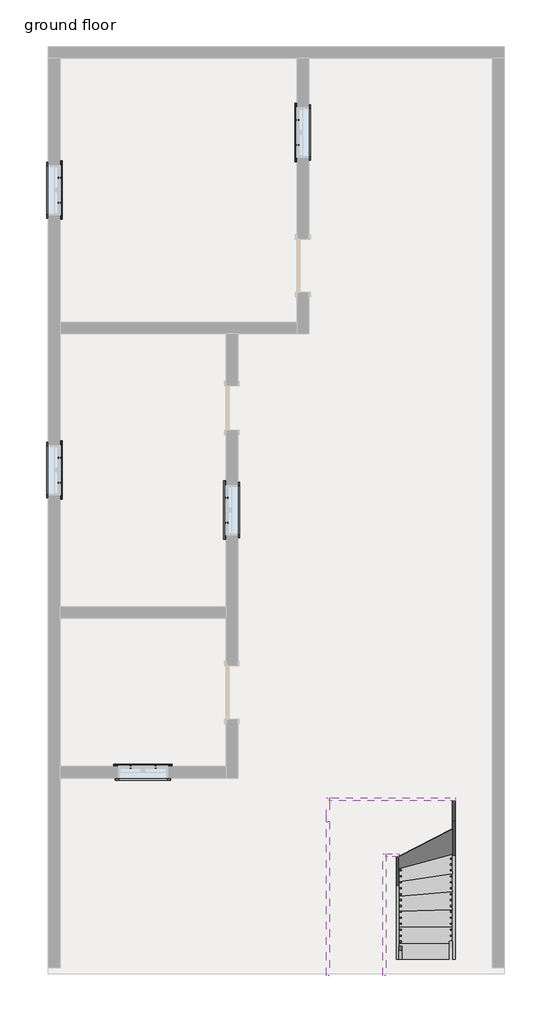
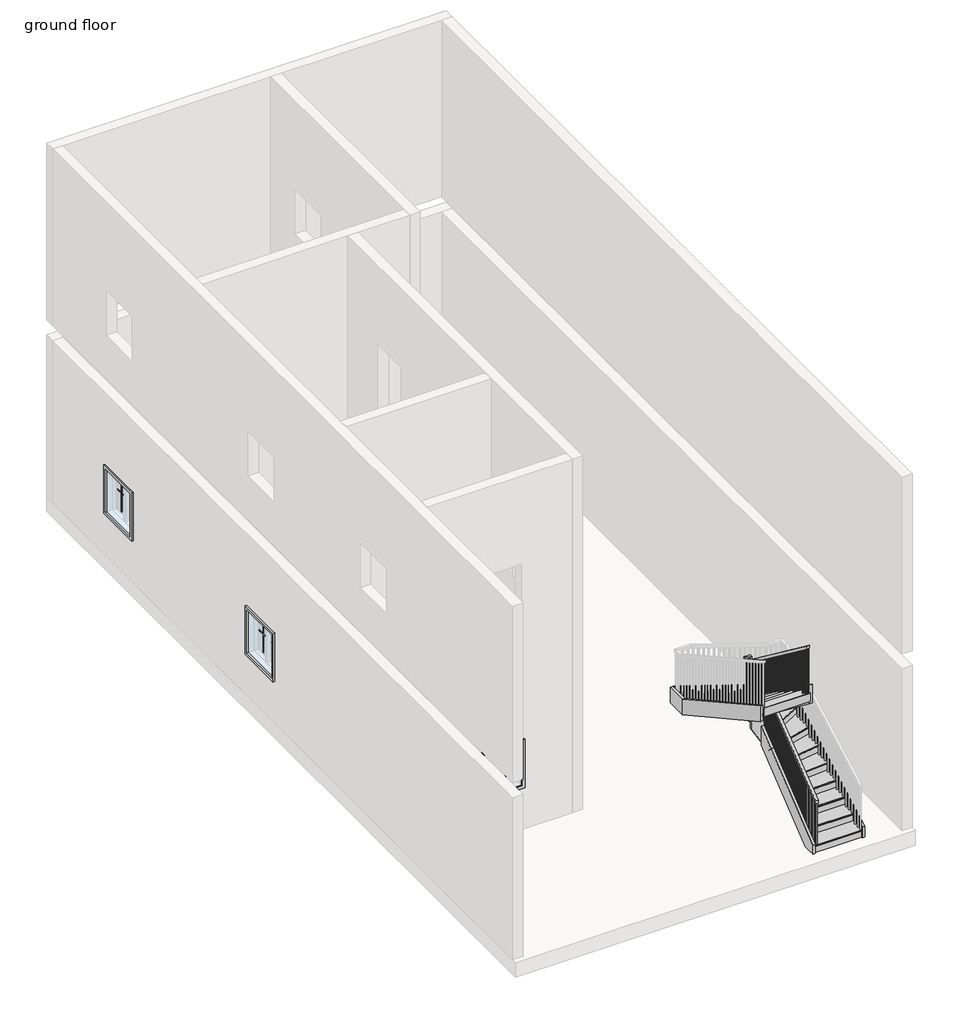
# One storey, part 2 of 2: 20 proxies, 8 members, 1 railing, 1 stair flight.
"""IFC4 building model written with IfcOpenShell, lengths in millimetres."""

from ifc_helpers import new_model, si_unit, frame, origin, place, context, project, spatial, polyline, outline, extrude, faceted_brep, transform, mapped, element, save
from components import muntin_pattern_2x2_muntin_pattern_2x2_b3fe6957, muntin_pattern_2x2_muntin_pattern_2x2_3e0ecaf2, trim_window_exterior_flat_with_sill_41619996, trim_window_exterior_flat_with_sill_f2223f96, trim_window_interior_flat_picture_frame_51c85655, trim_window_interior_flat_picture_frame_1c9020d0, stair_flight_39349fbd

model = new_model("IFC4")

# Units and contexts
model_context = context("Model", 3, world=origin())
ifc_project = project(units=[si_unit("LENGTHUNIT", "METRE", prefix="MILLI")], contexts=[model_context])

# Site, building, storey
site = spatial("IfcSite", under=ifc_project)
building = spatial("IfcBuilding", under=site)
storey = spatial("IfcBuildingStorey", under=building, Name="ground floor", Elevation=1828.8)

# Proxies
placement = place(None, origin())
muntin_pattern_2x2_muntin_pattern_2x2_shape = muntin_pattern_2x2_muntin_pattern_2x2_b3fe6957(model_context)
element("IfcBuildingElementProxy", 1, Name="Muntin Pattern_2x2 : Muntin Pattern_2x2", ObjectType="Muntin Pattern_2x2 : Muntin Pattern_2x2", at=placement, inside=storey, context=model_context, shape_type="MappedRepresentation", body=[
    mapped(muntin_pattern_2x2_muntin_pattern_2x2_shape, transform((-11607.3637549, 14376.3902962, 2813.05), x_axis=(0.0, 1.0, 0.0), y_axis=(-1.0, 0.0, 0.0), z_axis=(0.0, 0.0, 1.0))),
])
element("IfcBuildingElementProxy", 2, Name="Muntin Pattern_2x2 : Muntin Pattern_2x2", ObjectType="Muntin Pattern_2x2 : Muntin Pattern_2x2", at=placement, inside=storey, context=model_context, shape_type="MappedRepresentation", body=[
    mapped(muntin_pattern_2x2_muntin_pattern_2x2_shape, transform((-14472.8012549, 3709.9777962, 2813.05), x_axis=(1.0, 0.0, 0.0), y_axis=(0.0, 1.0, 0.0), z_axis=(0.0, 0.0, 1.0))),
])
element("IfcBuildingElementProxy", 3, Name="Muntin Pattern_2x2 : Muntin Pattern_2x2", ObjectType="Muntin Pattern_2x2 : Muntin Pattern_2x2", at=placement, inside=storey, context=model_context, shape_type="MappedRepresentation", body=[
    mapped(muntin_pattern_2x2_muntin_pattern_2x2_shape, transform((-12826.5637549, 7899.3902962, 2813.05), x_axis=(0.0, 1.0, 0.0), y_axis=(-1.0, 0.0, 0.0), z_axis=(0.0, 0.0, 1.0))),
])
element("IfcBuildingElementProxy", 4, Name="Muntin Pattern_2x2 : Muntin Pattern_2x2", ObjectType="Muntin Pattern_2x2 : Muntin Pattern_2x2", at=placement, inside=storey, context=model_context, shape_type="MappedRepresentation", body=[
    mapped(muntin_pattern_2x2_muntin_pattern_2x2_shape, transform((-15690.4137549, 13814.4152962, 2813.05), x_axis=(0.0, -1.0, 0.0), y_axis=(1.0, 0.0, 0.0), z_axis=(0.0, 0.0, 1.0))),
])
element("IfcBuildingElementProxy", 5, Name="Muntin Pattern_2x2 : Muntin Pattern_2x2", ObjectType="Muntin Pattern_2x2 : Muntin Pattern_2x2", at=placement, inside=storey, context=model_context, shape_type="MappedRepresentation", body=[
    mapped(muntin_pattern_2x2_muntin_pattern_2x2_shape, transform((-15690.4137549, 9013.8152962, 2813.05), x_axis=(0.0, -1.0, 0.0), y_axis=(1.0, 0.0, 0.0), z_axis=(0.0, 0.0, 1.0))),
])
muntin_pattern_2x2_muntin_pattern_2x2_2_shape = muntin_pattern_2x2_muntin_pattern_2x2_3e0ecaf2(model_context)
element("IfcBuildingElementProxy", 6, Name="Muntin Pattern_2x2 : Muntin Pattern_2x2", ObjectType="Muntin Pattern_2x2 : Muntin Pattern_2x2", at=placement, inside=storey, context=model_context, shape_type="MappedRepresentation", body=[
    mapped(muntin_pattern_2x2_muntin_pattern_2x2_2_shape, transform((-11607.3637549, 14805.0152962, 2813.05), x_axis=(0.0, -1.0, 0.0), y_axis=(1.0, 0.0, 0.0), z_axis=(0.0, 0.0, 1.0))),
])
element("IfcBuildingElementProxy", 7, Name="Muntin Pattern_2x2 : Muntin Pattern_2x2", ObjectType="Muntin Pattern_2x2 : Muntin Pattern_2x2", at=placement, inside=storey, context=model_context, shape_type="MappedRepresentation", body=[
    mapped(muntin_pattern_2x2_muntin_pattern_2x2_2_shape, transform((-14044.1762549, 3709.9777962, 2813.05), x_axis=(-1.0, 0.0, 0.0), y_axis=(0.0, -1.0, 0.0), z_axis=(0.0, 0.0, 1.0))),
])
element("IfcBuildingElementProxy", 8, Name="Muntin Pattern_2x2 : Muntin Pattern_2x2", ObjectType="Muntin Pattern_2x2 : Muntin Pattern_2x2", at=placement, inside=storey, context=model_context, shape_type="MappedRepresentation", body=[
    mapped(muntin_pattern_2x2_muntin_pattern_2x2_2_shape, transform((-12826.5637549, 8328.0152962, 2813.05), x_axis=(0.0, -1.0, 0.0), y_axis=(1.0, 0.0, 0.0), z_axis=(0.0, 0.0, 1.0))),
])
element("IfcBuildingElementProxy", 9, Name="Muntin Pattern_2x2 : Muntin Pattern_2x2", ObjectType="Muntin Pattern_2x2 : Muntin Pattern_2x2", at=placement, inside=storey, context=model_context, shape_type="MappedRepresentation", body=[
    mapped(muntin_pattern_2x2_muntin_pattern_2x2_2_shape, transform((-15690.4137549, 13385.7902962, 2813.05), x_axis=(0.0, 1.0, 0.0), y_axis=(-1.0, 0.0, 0.0), z_axis=(0.0, 0.0, 1.0))),
])
element("IfcBuildingElementProxy", 10, Name="Muntin Pattern_2x2 : Muntin Pattern_2x2", ObjectType="Muntin Pattern_2x2 : Muntin Pattern_2x2", at=placement, inside=storey, context=model_context, shape_type="MappedRepresentation", body=[
    mapped(muntin_pattern_2x2_muntin_pattern_2x2_2_shape, transform((-15690.4137549, 8585.1902962, 2813.05), x_axis=(0.0, 1.0, 0.0), y_axis=(-1.0, 0.0, 0.0), z_axis=(0.0, 0.0, 1.0))),
])
trim_window_exterior_flat_with_sill_shape = trim_window_exterior_flat_with_sill_41619996(model_context)
element("IfcBuildingElementProxy", 11, Name="Trim-Window-Exterior-Flat : with Sill", ObjectType="Trim-Window-Exterior-Flat : with Sill", at=placement, inside=storey, context=model_context, shape_type="MappedRepresentation", body=[
    mapped(trim_window_exterior_flat_with_sill_shape, transform((-14258.4887549, 3719.5027962, 3657.6), x_axis=(-1.0, 0.0, 0.0), y_axis=(0.0, 0.0, 1.0), z_axis=(0.0, 1.0, 0.0))),
])
element("IfcBuildingElementProxy", 12, Name="Trim-Window-Exterior-Flat : with Sill", ObjectType="Trim-Window-Exterior-Flat : with Sill", at=placement, inside=storey, context=model_context, shape_type="MappedRepresentation", body=[
    mapped(trim_window_exterior_flat_with_sill_shape, transform((-12836.0887549, 8113.7027962, 3657.6), x_axis=(0.0, -1.0, 0.0), y_axis=(0.0, 0.0, 1.0), z_axis=(-1.0, 0.0, 0.0))),
])
element("IfcBuildingElementProxy", 13, Name="Trim-Window-Exterior-Flat : with Sill", ObjectType="Trim-Window-Exterior-Flat : with Sill", at=placement, inside=storey, context=model_context, shape_type="MappedRepresentation", body=[
    mapped(trim_window_exterior_flat_with_sill_shape, transform((-15680.8887549, 13600.1027962, 3657.6), x_axis=(0.0, 1.0, 0.0), y_axis=(0.0, 0.0, 1.0), z_axis=(1.0, 0.0, 0.0))),
])
element("IfcBuildingElementProxy", 14, Name="Trim-Window-Exterior-Flat : with Sill", ObjectType="Trim-Window-Exterior-Flat : with Sill", at=placement, inside=storey, context=model_context, shape_type="MappedRepresentation", body=[
    mapped(trim_window_exterior_flat_with_sill_shape, transform((-15680.8887549, 8799.5027962, 3657.6), x_axis=(0.0, 1.0, 0.0), y_axis=(0.0, 0.0, 1.0), z_axis=(1.0, 0.0, 0.0))),
])
trim_window_exterior_flat_with_sill_2_shape = trim_window_exterior_flat_with_sill_f2223f96(model_context)
element("IfcBuildingElementProxy", 15, Name="Trim-Window-Exterior-Flat : with Sill", ObjectType="Trim-Window-Exterior-Flat : with Sill", at=placement, inside=storey, context=model_context, shape_type="MappedRepresentation", body=[
    mapped(trim_window_exterior_flat_with_sill_2_shape, transform((-11616.8887549, 14590.7027962, 3657.6), x_axis=(0.0, 1.0, 0.0), y_axis=(0.0, 0.0, -1.0), z_axis=(-1.0, 0.0, 0.0))),
])
trim_window_interior_flat_picture_frame_shape = trim_window_interior_flat_picture_frame_51c85655(model_context)
element("IfcBuildingElementProxy", 16, Name="Trim-Window-Interior-Flat : Picture Frame", ObjectType="Trim-Window-Interior-Flat : Picture Frame", at=placement, inside=storey, context=model_context, shape_type="MappedRepresentation", body=[
    mapped(trim_window_interior_flat_picture_frame_shape, transform((-14258.4887549, 3516.3027962, 3657.6), x_axis=(1.0, 0.0, 0.0), y_axis=(0.0, 0.0, 1.0), z_axis=(0.0, -1.0, 0.0))),
])
element("IfcBuildingElementProxy", 17, Name="Trim-Window-Interior-Flat : Picture Frame", ObjectType="Trim-Window-Interior-Flat : Picture Frame", at=placement, inside=storey, context=model_context, shape_type="MappedRepresentation", body=[
    mapped(trim_window_interior_flat_picture_frame_shape, transform((-12632.8887549, 8113.7027962, 3657.6), x_axis=(0.0, 1.0, 0.0), y_axis=(0.0, 0.0, 1.0), z_axis=(1.0, 0.0, 0.0))),
])
element("IfcBuildingElementProxy", 18, Name="Trim-Window-Interior-Flat : Picture Frame", ObjectType="Trim-Window-Interior-Flat : Picture Frame", at=placement, inside=storey, context=model_context, shape_type="MappedRepresentation", body=[
    mapped(trim_window_interior_flat_picture_frame_shape, transform((-15884.0887549, 13600.1027962, 3657.6), x_axis=(0.0, -1.0, 0.0), y_axis=(0.0, 0.0, 1.0), z_axis=(-1.0, 0.0, 0.0))),
])
element("IfcBuildingElementProxy", 19, Name="Trim-Window-Interior-Flat : Picture Frame", ObjectType="Trim-Window-Interior-Flat : Picture Frame", at=placement, inside=storey, context=model_context, shape_type="MappedRepresentation", body=[
    mapped(trim_window_interior_flat_picture_frame_shape, transform((-15884.0887549, 8799.5027962, 3657.6), x_axis=(0.0, -1.0, 0.0), y_axis=(0.0, 0.0, 1.0), z_axis=(-1.0, 0.0, 0.0))),
])
trim_window_interior_flat_picture_frame_2_shape = trim_window_interior_flat_picture_frame_1c9020d0(model_context)
element("IfcBuildingElementProxy", 20, Name="Trim-Window-Interior-Flat : Picture Frame", ObjectType="Trim-Window-Interior-Flat : Picture Frame", at=placement, inside=storey, context=model_context, shape_type="MappedRepresentation", body=[
    mapped(trim_window_interior_flat_picture_frame_2_shape, transform((-11413.6887549, 14590.7027962, 3657.6), x_axis=(0.0, -1.0, 0.0), y_axis=(0.0, 0.0, -1.0), z_axis=(1.0, 0.0, 0.0))),
])

# Members
element("IfcMember", 21, ObjectType="Stringer - 2\" Width", at=placement, inside=storey, context=model_context, shape_type="SweptSolid", body=[
    extrude(outline(polyline([(413.7711043, 1828.8), (413.7711043, 2012.3893785), (2170.1027962, 3416.1064752), (2170.1027962, 3025.9181459), (672.2678383, 1828.8), (413.7711043, 1828.8)])), frame((-9915.0887549, 0.0, 0.0), z_axis=(1.0, 0.0, 0.0), x_axis=(0.0, 1.0, 0.0)), (0.0, 0.0, 1.0), 50.8),
])
element("IfcMember", 22, ObjectType="Stringer - 2\" Width", at=placement, inside=storey, context=model_context, shape_type="SweptSolid", body=[
    extrude(outline(polyline([(3066.519149, -9864.2887549), (3619.1941419, -9864.2887549), (3972.4646785, -10065.4124649), (3972.4646785, -10092.8887549), (3404.6656421, -10092.8887549), (3066.519149, -9900.3754537), (3066.519149, -9864.2887549)])), frame((0.0, 2170.1027962, 0.0), z_axis=(0.0, 1.0, 0.0), x_axis=(0.0, 0.0, 1.0)), (0.0, 0.0, 1.0), 50.8),
])
element("IfcMember", 23, ObjectType="Stringer - 2\" Width", at=placement, inside=storey, context=model_context, shape_type="SweptSolid", body=[
    extrude(outline(polyline([(2220.9027962, 3972.4646785), (2220.9027962, 3587.4022375), (134.3711043, 5198.2238766), (134.3711043, 5583.2863176), (2220.9027962, 3972.4646785)])), frame((-10143.6887549, 0.0, 0.0), z_axis=(1.0, 0.0, 0.0), x_axis=(0.0, 1.0, 0.0)), (0.0, 0.0, 1.0), 50.8),
])
element("IfcMember", 24, ObjectType="Stringer - 2\" Width", at=placement, inside=storey, context=model_context, shape_type="SweptSolid", body=[
    extrude(outline(polyline([(413.7711043, 1828.8), (413.7711043, 2057.6707329), (2776.4692037, 3342.1226437), (2776.4692037, 2995.1935559), (630.934743, 1828.8), (413.7711043, 1828.8)])), frame((-8949.8887549, 0.0, 0.0), z_axis=(1.0, 0.0, 0.0), x_axis=(0.0, 1.0, 0.0)), (0.0, 0.0, 1.0), 50.8),
])
element("IfcMember", 25, ObjectType="Stringer - 2\" Width", at=placement, inside=storey, context=model_context, shape_type="SweptSolid", body=[
    extrude(outline(polyline([(-8899.0887549, 2776.4692037), (-8949.8887549, 2776.4692037), (-8949.8887549, 3135.3027962), (-8899.0887549, 3135.3027962), (-8899.0887549, 2776.4692037)])), frame((0.0, 0.0, 2995.1935559), z_axis=(0.0, 0.0, 1.0), x_axis=(1.0, 0.0, 0.0)), (0.0, 0.0, 1.0), 346.9290877),
])
element("IfcMember", 26, ObjectType="Stringer - 2\" Width", at=placement, inside=storey, context=model_context, shape_type="SweptSolid", body=[
    extrude(outline(polyline([(3037.3226437, -8899.0887549), (3325.3564932, -8899.0887549), (4024.1498782, -11016.3728581), (4024.1498782, -11058.0887549), (3690.9888024, -11058.0887549), (3037.3226437, -9077.5362822), (3037.3226437, -8899.0887549)])), frame((0.0, 3135.3027962, 0.0), z_axis=(0.0, 1.0, 0.0), x_axis=(0.0, 0.0, 1.0)), (0.0, 0.0, 1.0), 50.8),
])
element("IfcMember", 27, ObjectType="Stringer - 2\" Width", at=placement, inside=storey, context=model_context, shape_type="SweptSolid", body=[
    extrude(outline(polyline([(-11108.8887549, 3186.1027962), (-11058.0887549, 3186.1027962), (-11058.0887549, 2773.526995), (-11108.8887549, 2773.526995), (-11108.8887549, 3186.1027962)])), frame((0.0, 0.0, 3703.1782644), z_axis=(0.0, 0.0, 1.0), x_axis=(1.0, 0.0, 0.0)), (0.0, 0.0, 1.0), 320.9716139),
])
element("IfcMember", 28, ObjectType="Stringer - 2\" Width", at=placement, inside=storey, context=model_context, shape_type="SweptSolid", body=[
    extrude(outline(polyline([(2773.526995, 4024.1498782), (2773.526995, 3703.1782644), (134.3711043, 5164.6288716), (134.3711043, 5485.6004855), (2773.526995, 4024.1498782)])), frame((-11108.8887549, 0.0, 0.0), z_axis=(1.0, 0.0, 0.0), x_axis=(0.0, 1.0, 0.0)), (0.0, 0.0, 1.0), 50.8),
])

# Railing
element("IfcRailing", 29, ObjectType="Handrail - Rectangular", at=placement, inside=storey, context=model_context, shape_type="SolidModel", body=[
    faceted_brep([(-9864.2887549, 413.7711043, 2917.3714286), (-9864.2887549, 413.7711043, 2853.1943551), (-9813.4887549, 413.7711043, 2853.1943551), (-9813.4887549, 413.7711043, 2917.3714286), (-9864.2887549, 2144.7027962, 4253.6666001), (-9864.2887549, 2195.5027962, 4228.7075934), (-9813.4887549, 2195.5027962, 4228.7075934), (-9813.4887549, 2144.7027962, 4253.6666001), (-9970.0232047, 2220.9027962, 4409.6632793), (-9940.4887549, 2220.9027962, 4460.4632793), (-10067.4887549, 2220.9027962, 4683.5367207), (-10118.2887549, 2220.9027962, 4670.0893149), (-9970.0232047, 2271.7027962, 4409.6632793), (-10118.2887549, 2271.7027962, 4670.0893149), (-9940.4887549, 2271.7027962, 4460.4632793), (-10067.4887549, 2271.7027962, 4683.5367207), (-10143.6887549, 134.3711043, 6400.8), (-10194.4887549, 134.3711043, 6400.8), (-10194.4887549, 134.3711043, 6337.2364026), (-10143.6887549, 134.3711043, 6337.2364026), (-10143.6887549, 2127.7318382, 4838.060339), (-10143.6887549, 2144.7027962, 4888.860339), (-10194.4887549, 2127.7318382, 4838.060339), (-10194.4887549, 2144.7027962, 4888.860339), (-9864.2887549, 2144.7027962, 4460.4632793), (-9864.2887549, 2195.5027962, 4409.6632793), (-9813.4887549, 2195.5027962, 4409.6632793), (-9813.4887549, 2144.7027962, 4460.4632793), (-9864.2887549, 2220.9027962, 4460.4632793), (-9864.2887549, 2220.9027962, 4409.6632793), (-9813.4887549, 2271.7027962, 4409.6632793), (-9813.4887549, 2271.7027962, 4460.4632793), (-10067.4887549, 2220.9027962, 4888.860339), (-10118.2887549, 2220.9027962, 4838.060339), (-10118.2887549, 2271.7027962, 4838.060339), (-10067.4887549, 2271.7027962, 4888.860339), (-10143.6887549, 2220.9027962, 4888.860339), (-10143.6887549, 2220.9027962, 4838.060339), (-10194.4887549, 2271.7027962, 4838.060339), (-10194.4887549, 2271.7027962, 4888.860339)], [[[0, 1, 2, 3]], [[1, 0, 4, 5]], [[2, 1, 5, 6]], [[3, 2, 6, 7]], [[0, 3, 7, 4]], [[8, 9, 10, 11]], [[12, 8, 11, 13]], [[14, 12, 13, 15]], [[9, 14, 15, 10]], [[16, 17, 18, 19]], [[20, 21, 16, 19]], [[22, 20, 19, 18]], [[23, 22, 18, 17]], [[21, 23, 17, 16]], [[5, 4, 24, 25]], [[6, 5, 25, 26]], [[7, 6, 26, 27]], [[4, 7, 27, 24]], [[25, 24, 28, 29]], [[26, 25, 29, 30]], [[27, 26, 30, 31]], [[24, 27, 31, 28]], [[29, 28, 9, 8]], [[30, 29, 8, 12]], [[31, 30, 12, 14]], [[28, 31, 14, 9]], [[11, 10, 32, 33]], [[13, 11, 33, 34]], [[15, 13, 34, 35]], [[10, 15, 35, 32]], [[33, 32, 36, 37]], [[34, 33, 37, 38]], [[35, 34, 38, 39]], [[32, 35, 39, 36]], [[37, 36, 21, 20]], [[38, 37, 20, 22]], [[39, 38, 22, 23]], [[36, 39, 23, 21]]]),
    extrude(outline(polyline([(223.8277962, 6269.9573954), (223.8277962, 5312.2285714), (204.7777962, 5312.2285714), (204.7777962, 6284.2846085), (223.8277962, 6269.9573954)])), frame((-10178.6137549, 0.0, 0.0), z_axis=(1.0, 0.0, 0.0), x_axis=(0.0, 1.0, 0.0)), (0.0, 0.0, 1.0), 19.05),
    extrude(outline(polyline([(325.4277962, 6193.5455922), (325.4277962, 5312.2285714), (306.3777962, 5312.2285714), (306.3777962, 6207.8728053), (325.4277962, 6193.5455922)])), frame((-10178.6137549, 0.0, 0.0), z_axis=(1.0, 0.0, 0.0), x_axis=(0.0, 1.0, 0.0)), (0.0, 0.0, 1.0), 19.05),
    extrude(outline(polyline([(427.0277962, 6117.133789), (427.0277962, 5138.0571429), (407.9777962, 5138.0571429), (407.9777962, 6131.4610021), (427.0277962, 6117.133789)])), frame((-10178.6137549, 0.0, 0.0), z_axis=(1.0, 0.0, 0.0), x_axis=(0.0, 1.0, 0.0)), (0.0, 0.0, 1.0), 19.05),
    extrude(outline(polyline([(528.6277962, 6040.7219859), (528.6277962, 5138.0571429), (509.5777962, 5138.0571429), (509.5777962, 6055.049199), (528.6277962, 6040.7219859)])), frame((-10178.6137549, 0.0, 0.0), z_axis=(1.0, 0.0, 0.0), x_axis=(0.0, 1.0, 0.0)), (0.0, 0.0, 1.0), 19.05),
    extrude(outline(polyline([(630.2277962, 5964.3101827), (630.2277962, 5138.0571429), (611.1777962, 5138.0571429), (611.1777962, 5978.6373958), (630.2277962, 5964.3101827)])), frame((-10178.6137549, 0.0, 0.0), z_axis=(1.0, 0.0, 0.0), x_axis=(0.0, 1.0, 0.0)), (0.0, 0.0, 1.0), 19.05),
    extrude(outline(polyline([(731.8277962, 5887.8983795), (731.8277962, 4963.8857143), (712.7777962, 4963.8857143), (712.7777962, 5902.2255926), (731.8277962, 5887.8983795)])), frame((-10178.6137549, 0.0, 0.0), z_axis=(1.0, 0.0, 0.0), x_axis=(0.0, 1.0, 0.0)), (0.0, 0.0, 1.0), 19.05),
    extrude(outline(polyline([(833.4277962, 5811.4865763), (833.4277962, 4963.8857143), (814.3777962, 4963.8857143), (814.3777962, 5825.8137894), (833.4277962, 5811.4865763)])), frame((-10178.6137549, 0.0, 0.0), z_axis=(1.0, 0.0, 0.0), x_axis=(0.0, 1.0, 0.0)), (0.0, 0.0, 1.0), 19.05),
    extrude(outline(polyline([(935.0277962, 5735.0747731), (935.0277962, 4963.8857143), (915.9777962, 4963.8857143), (915.9777962, 5749.4019862), (935.0277962, 5735.0747731)])), frame((-10178.6137549, 0.0, 0.0), z_axis=(1.0, 0.0, 0.0), x_axis=(0.0, 1.0, 0.0)), (0.0, 0.0, 1.0), 19.05),
    extrude(outline(polyline([(1036.6277962, 5658.66297), (1036.6277962, 4789.7142857), (1017.5777962, 4789.7142857), (1017.5777962, 5672.9901831), (1036.6277962, 5658.66297)])), frame((-10178.6137549, 0.0, 0.0), z_axis=(1.0, 0.0, 0.0), x_axis=(0.0, 1.0, 0.0)), (0.0, 0.0, 1.0), 19.05),
    extrude(outline(polyline([(1138.2277962, 5582.2511668), (1138.2277962, 4789.7142857), (1119.1777962, 4789.7142857), (1119.1777962, 5596.5783799), (1138.2277962, 5582.2511668)])), frame((-10178.6137549, 0.0, 0.0), z_axis=(1.0, 0.0, 0.0), x_axis=(0.0, 1.0, 0.0)), (0.0, 0.0, 1.0), 19.05),
    extrude(outline(polyline([(1239.8277962, 5505.8393636), (1239.8277962, 4615.5428571), (1220.7777962, 4615.5428571), (1220.7777962, 5520.1665767), (1239.8277962, 5505.8393636)])), frame((-10178.6137549, 0.0, 0.0), z_axis=(1.0, 0.0, 0.0), x_axis=(0.0, 1.0, 0.0)), (0.0, 0.0, 1.0), 19.05),
    extrude(outline(polyline([(1341.4277962, 5429.4275604), (1341.4277962, 4615.5428571), (1322.3777962, 4615.5428571), (1322.3777962, 5443.7547735), (1341.4277962, 5429.4275604)])), frame((-10178.6137549, 0.0, 0.0), z_axis=(1.0, 0.0, 0.0), x_axis=(0.0, 1.0, 0.0)), (0.0, 0.0, 1.0), 19.05),
    extrude(outline(polyline([(1443.0277962, 5353.0157573), (1443.0277962, 4615.5428571), (1423.9777962, 4615.5428571), (1423.9777962, 5367.3429704), (1443.0277962, 5353.0157573)])), frame((-10178.6137549, 0.0, 0.0), z_axis=(1.0, 0.0, 0.0), x_axis=(0.0, 1.0, 0.0)), (0.0, 0.0, 1.0), 19.05),
    extrude(outline(polyline([(1544.6277962, 5276.6039541), (1544.6277962, 4441.3714286), (1525.5777962, 4441.3714286), (1525.5777962, 5290.9311672), (1544.6277962, 5276.6039541)])), frame((-10178.6137549, 0.0, 0.0), z_axis=(1.0, 0.0, 0.0), x_axis=(0.0, 1.0, 0.0)), (0.0, 0.0, 1.0), 19.05),
    extrude(outline(polyline([(1646.2277962, 5200.1921509), (1646.2277962, 4441.3714286), (1627.1777962, 4441.3714286), (1627.1777962, 5214.519364), (1646.2277962, 5200.1921509)])), frame((-10178.6137549, 0.0, 0.0), z_axis=(1.0, 0.0, 0.0), x_axis=(0.0, 1.0, 0.0)), (0.0, 0.0, 1.0), 19.05),
    extrude(outline(polyline([(1747.8277962, 5123.7803477), (1747.8277962, 4441.3714286), (1728.7777962, 4441.3714286), (1728.7777962, 5138.1075608), (1747.8277962, 5123.7803477)])), frame((-10178.6137549, 0.0, 0.0), z_axis=(1.0, 0.0, 0.0), x_axis=(0.0, 1.0, 0.0)), (0.0, 0.0, 1.0), 19.05),
    extrude(outline(polyline([(1849.4277962, 5047.3685445), (1849.4277962, 4267.2), (1830.3777962, 4267.2), (1830.3777962, 5061.6957576), (1849.4277962, 5047.3685445)])), frame((-10178.6137549, 0.0, 0.0), z_axis=(1.0, 0.0, 0.0), x_axis=(0.0, 1.0, 0.0)), (0.0, 0.0, 1.0), 19.05),
    extrude(outline(polyline([(1951.0277962, 4970.9567414), (1951.0277962, 4267.2), (1931.9777962, 4267.2), (1931.9777962, 4985.2839545), (1951.0277962, 4970.9567414)])), frame((-10178.6137549, 0.0, 0.0), z_axis=(1.0, 0.0, 0.0), x_axis=(0.0, 1.0, 0.0)), (0.0, 0.0, 1.0), 19.05),
    extrude(outline(polyline([(2052.6277962, 4894.5449382), (2052.6277962, 4093.0285714), (2033.5777962, 4093.0285714), (2033.5777962, 4908.8721513), (2052.6277962, 4894.5449382)])), frame((-10178.6137549, 0.0, 0.0), z_axis=(1.0, 0.0, 0.0), x_axis=(0.0, 1.0, 0.0)), (0.0, 0.0, 1.0), 19.05),
    extrude(outline(polyline([(2154.2277962, 4818.133135), (2154.2277962, 4093.0285714), (2135.1777962, 4093.0285714), (2135.1777962, 4832.4603481), (2154.2277962, 4818.133135)])), frame((-10178.6137549, 0.0, 0.0), z_axis=(1.0, 0.0, 0.0), x_axis=(0.0, 1.0, 0.0)), (0.0, 0.0, 1.0), 19.05),
    extrude(outline(polyline([(-10134.1637549, 2236.7777962), (-10153.2137549, 2236.7777962), (-10153.2137549, 2255.8277962), (-10134.1637549, 2255.8277962), (-10134.1637549, 2236.7777962)])), frame((0.0, 0.0, 3744.6857143), z_axis=(0.0, 0.0, 1.0), x_axis=(1.0, 0.0, 0.0)), (0.0, 0.0, 1.0), 1093.3746247),
    extrude(outline(polyline([(4552.9757581, -10051.6137549), (3570.5142857, -10051.6137549), (3570.5142857, -10032.5637549), (4519.5147419, -10032.5637549), (4552.9757581, -10051.6137549)])), frame((0.0, 2236.7777962, 0.0), z_axis=(0.0, 1.0, 0.0), x_axis=(0.0, 0.0, 1.0)), (0.0, 0.0, 1.0), 19.05),
    extrude(outline(polyline([(4374.517005, -9950.0137549), (3396.3428571, -9950.0137549), (3396.3428571, -9930.9637549), (4341.0559888, -9930.9637549), (4374.517005, -9950.0137549)])), frame((0.0, 2236.7777962, 0.0), z_axis=(0.0, 1.0, 0.0), x_axis=(0.0, 0.0, 1.0)), (0.0, 0.0, 1.0), 19.05),
    extrude(outline(polyline([(-9848.4137549, 2233.0461043), (-9848.4137549, 2252.0961043), (-9829.3637549, 2252.0961043), (-9829.3637549, 2233.0461043), (-9848.4137549, 2233.0461043)])), frame((0.0, 0.0, 3222.1714286), z_axis=(0.0, 0.0, 1.0), x_axis=(1.0, 0.0, 0.0)), (0.0, 0.0, 1.0), 1187.4918507),
    extrude(outline(polyline([(2150.4961043, 4193.9620137), (2150.4961043, 3048.0), (2131.4461043, 3048.0), (2131.4461043, 4179.2552387), (2150.4961043, 4193.9620137)])), frame((-9848.4137549, 0.0, 0.0), z_axis=(1.0, 0.0, 0.0), x_axis=(0.0, 1.0, 0.0)), (0.0, 0.0, 1.0), 19.05),
    extrude(outline(polyline([(2048.8961043, 4115.5258801), (2048.8961043, 3048.0), (2029.8461043, 3048.0), (2029.8461043, 4100.8191051), (2048.8961043, 4115.5258801)])), frame((-9848.4137549, 0.0, 0.0), z_axis=(1.0, 0.0, 0.0), x_axis=(0.0, 1.0, 0.0)), (0.0, 0.0, 1.0), 19.05),
    extrude(outline(polyline([(1947.2961043, 4037.0897465), (1947.2961043, 2873.8285714), (1928.2461043, 2873.8285714), (1928.2461043, 4022.3829715), (1947.2961043, 4037.0897465)])), frame((-9848.4137549, 0.0, 0.0), z_axis=(1.0, 0.0, 0.0), x_axis=(0.0, 1.0, 0.0)), (0.0, 0.0, 1.0), 19.05),
    extrude(outline(polyline([(1845.6961043, 3958.6536129), (1845.6961043, 2873.8285714), (1826.6461043, 2873.8285714), (1826.6461043, 3943.9468379), (1845.6961043, 3958.6536129)])), frame((-9848.4137549, 0.0, 0.0), z_axis=(1.0, 0.0, 0.0), x_axis=(0.0, 1.0, 0.0)), (0.0, 0.0, 1.0), 19.05),
    extrude(outline(polyline([(1744.0961043, 3880.2174793), (1744.0961043, 2699.6571429), (1725.0461043, 2699.6571429), (1725.0461043, 3865.5107043), (1744.0961043, 3880.2174793)])), frame((-9848.4137549, 0.0, 0.0), z_axis=(1.0, 0.0, 0.0), x_axis=(0.0, 1.0, 0.0)), (0.0, 0.0, 1.0), 19.05),
    extrude(outline(polyline([(1642.4961043, 3801.7813457), (1642.4961043, 2699.6571429), (1623.4461043, 2699.6571429), (1623.4461043, 3787.0745707), (1642.4961043, 3801.7813457)])), frame((-9848.4137549, 0.0, 0.0), z_axis=(1.0, 0.0, 0.0), x_axis=(0.0, 1.0, 0.0)), (0.0, 0.0, 1.0), 19.05),
    extrude(outline(polyline([(1540.8961043, 3723.3452121), (1540.8961043, 2699.6571429), (1521.8461043, 2699.6571429), (1521.8461043, 3708.6384371), (1540.8961043, 3723.3452121)])), frame((-9848.4137549, 0.0, 0.0), z_axis=(1.0, 0.0, 0.0), x_axis=(0.0, 1.0, 0.0)), (0.0, 0.0, 1.0), 19.05),
    extrude(outline(polyline([(1439.2961043, 3644.9090785), (1439.2961043, 2525.4857143), (1420.2461043, 2525.4857143), (1420.2461043, 3630.2023035), (1439.2961043, 3644.9090785)])), frame((-9848.4137549, 0.0, 0.0), z_axis=(1.0, 0.0, 0.0), x_axis=(0.0, 1.0, 0.0)), (0.0, 0.0, 1.0), 19.05),
    extrude(outline(polyline([(1337.6961043, 3566.472945), (1337.6961043, 2525.4857143), (1318.6461043, 2525.4857143), (1318.6461043, 3551.7661699), (1337.6961043, 3566.472945)])), frame((-9848.4137549, 0.0, 0.0), z_axis=(1.0, 0.0, 0.0), x_axis=(0.0, 1.0, 0.0)), (0.0, 0.0, 1.0), 19.05),
    extrude(outline(polyline([(1236.0961043, 3488.0368114), (1236.0961043, 2351.3142857), (1217.0461043, 2351.3142857), (1217.0461043, 3473.3300363), (1236.0961043, 3488.0368114)])), frame((-9848.4137549, 0.0, 0.0), z_axis=(1.0, 0.0, 0.0), x_axis=(0.0, 1.0, 0.0)), (0.0, 0.0, 1.0), 19.05),
    extrude(outline(polyline([(1134.4961043, 3409.6006778), (1134.4961043, 2351.3142857), (1115.4461043, 2351.3142857), (1115.4461043, 3394.8939027), (1134.4961043, 3409.6006778)])), frame((-9848.4137549, 0.0, 0.0), z_axis=(1.0, 0.0, 0.0), x_axis=(0.0, 1.0, 0.0)), (0.0, 0.0, 1.0), 19.05),
    extrude(outline(polyline([(1032.8961043, 3331.1645442), (1032.8961043, 2351.3142857), (1013.8461043, 2351.3142857), (1013.8461043, 3316.4577691), (1032.8961043, 3331.1645442)])), frame((-9848.4137549, 0.0, 0.0), z_axis=(1.0, 0.0, 0.0), x_axis=(0.0, 1.0, 0.0)), (0.0, 0.0, 1.0), 19.05),
    extrude(outline(polyline([(931.2961043, 3252.7284106), (931.2961043, 2177.1428571), (912.2461043, 2177.1428571), (912.2461043, 3238.0216355), (931.2961043, 3252.7284106)])), frame((-9848.4137549, 0.0, 0.0), z_axis=(1.0, 0.0, 0.0), x_axis=(0.0, 1.0, 0.0)), (0.0, 0.0, 1.0), 19.05),
    extrude(outline(polyline([(829.6961043, 3174.292277), (829.6961043, 2177.1428571), (810.6461043, 2177.1428571), (810.6461043, 3159.5855019), (829.6961043, 3174.292277)])), frame((-9848.4137549, 0.0, 0.0), z_axis=(1.0, 0.0, 0.0), x_axis=(0.0, 1.0, 0.0)), (0.0, 0.0, 1.0), 19.05),
    extrude(outline(polyline([(728.0961043, 3095.8561434), (728.0961043, 2177.1428571), (709.0461043, 2177.1428571), (709.0461043, 3081.1493683), (728.0961043, 3095.8561434)])), frame((-9848.4137549, 0.0, 0.0), z_axis=(1.0, 0.0, 0.0), x_axis=(0.0, 1.0, 0.0)), (0.0, 0.0, 1.0), 19.05),
    extrude(outline(polyline([(626.4961043, 3017.4200098), (626.4961043, 2002.9714286), (607.4461043, 2002.9714286), (607.4461043, 3002.7132347), (626.4961043, 3017.4200098)])), frame((-9848.4137549, 0.0, 0.0), z_axis=(1.0, 0.0, 0.0), x_axis=(0.0, 1.0, 0.0)), (0.0, 0.0, 1.0), 19.05),
    extrude(outline(polyline([(524.8961043, 2938.9838762), (524.8961043, 2002.9714286), (505.8461043, 2002.9714286), (505.8461043, 2924.2771011), (524.8961043, 2938.9838762)])), frame((-9848.4137549, 0.0, 0.0), z_axis=(1.0, 0.0, 0.0), x_axis=(0.0, 1.0, 0.0)), (0.0, 0.0, 1.0), 19.05),
    extrude(outline(polyline([(-10159.5637549, 2236.7777962), (-10178.6137549, 2236.7777962), (-10178.6137549, 2255.8277962), (-10159.5637549, 2255.8277962), (-10159.5637549, 2236.7777962)])), frame((0.0, 0.0, 3918.8571429), z_axis=(0.0, 0.0, 1.0), x_axis=(1.0, 0.0, 0.0)), (0.0, 0.0, 1.0), 919.2031961),
    extrude(outline(polyline([(-9848.4137549, 2236.7777962), (-9848.4137549, 2255.8277962), (-9829.3637549, 2255.8277962), (-9829.3637549, 2236.7777962), (-9848.4137549, 2236.7777962)])), frame((0.0, 0.0, 3222.1714286), z_axis=(0.0, 0.0, 1.0), x_axis=(1.0, 0.0, 0.0)), (0.0, 0.0, 1.0), 1187.4918507),
    extrude(outline(polyline([(153.4211043, 6322.9091895), (153.4211043, 5312.2285714), (134.3711043, 5312.2285714), (134.3711043, 6337.2364026), (153.4211043, 6322.9091895)])), frame((-10178.6137549, 0.0, 0.0), z_axis=(1.0, 0.0, 0.0), x_axis=(0.0, 1.0, 0.0)), (0.0, 0.0, 1.0), 19.05),
    extrude(outline(polyline([(432.8211043, 2867.9011301), (432.8211043, 2002.9714286), (413.7711043, 2002.9714286), (413.7711043, 2853.1943551), (432.8211043, 2867.9011301)])), frame((-9848.4137549, 0.0, 0.0), z_axis=(1.0, 0.0, 0.0), x_axis=(0.0, 1.0, 0.0)), (0.0, 0.0, 1.0), 19.05),
])

# Stair flight
stair_flight_shape = stair_flight_39349fbd(model_context)
element("IfcStairFlight", 30, ObjectType="2\" Tread 1\" Nosing 1/4\" Riser", at=placement, inside=storey, context=model_context, shape_type="MappedRepresentation", body=[
    mapped(stair_flight_shape, transform((0.0, 0.0, 0.0), x_axis=(1.0, 0.0, 0.0), y_axis=(0.0, 1.0, 0.0), z_axis=(0.0, 0.0, 1.0))),
])

save(model, "model.ifc")

# Revit data of these elements
# Type "Muntin Pattern_2x2 : Muntin Pattern_2x2"
#   Width [instance default] = 4' - 0"
#   Thickness = 0' - 0 1/2"
#   Height [instance default] = 4' - 0"
#   Distance = 0' - 0 3/4"
#   Interior Material [instance default] = none
#   Exterior Material [instance default] = none
#   Default Elevation = 0
# Type "Trim-Window-Exterior-Flat : with Sill"
#   Trim Width = 0' - 2 1/4"
#   Trim Thickness_Picture Frame = 0' - 1 1/4"
#   Trim Thickness_with Sill = 0' - 0 3/4"
#   Sill Thickness = 0' - 1 1/4"
#   Opening Width [instance default] = 2' - 0"
#   Opening Height [instance default] = 3' - 0"
#   Default Elevation = 4' - 0"
#   Sill = yes
#   Picture Frame = no
#   Trim Material [instance default] = none
# Type "Trim-Window-Interior-Flat : Picture Frame"
#   Trim Thickness_Picture Frame = 0' - 1 1/4"
#   Trim Width = 0' - 2 1/4"
#   Trim Thickness_with Sill = 0' - 0 3/4"
#   Sill Thickness = 0' - 1 1/4"
#   Opening Width [instance default] = 2' - 0"
#   Opening Height [instance default] = 3' - 0"
#   Default Elevation = 4' - 0"
#   Sill = no
#   Picture Frame = yes
#   Trim Material [instance default] = none
# Type "Handrail - Rectangular"
#   Assembly Code = "C2010400"
#   built-in parameter 1008612 = 0.0416667 (stored number, unit not read)
#   built-in parameter 1008611 = 0.0416667 (stored number, unit not read)
#   built-in parameter 1008609 = 0.333333 (stored number, unit not read)
#   built-in parameter 1008604 = 0.166667 (stored number, unit not read)
#   built-in parameter 1008603 = 0.166667 (stored number, unit not read)
#   Railing Height = 3' - 0"
#   built-in parameter 1008630 = 2
#   built-in parameter 1008610 = 2
#   built-in parameter 1008618 = Baluster - Square : 3/4"
# Elements 1, 2, 3, 4, 5, 6, 7, 8, 9, 10 (IfcBuildingElementProxy, "Muntin Pattern_2x2 : Muntin Pattern_2x2")
#   Width = 0' - 11 5/8"
#   Height = 2' - 6 1/2"
#   Interior Material = Wood - Stained
#   Exterior Material = Clad - White
#   Phase Created = New Construction
#   Materials on its faces: "Clad - White", "Wood - Stained"
# Elements 11, 12, 13, 14, 15 (IfcBuildingElementProxy, "Trim-Window-Exterior-Flat : with Sill")
#   Opening Width = 2' - 10"
#   Opening Height = 3' - 0"
#   Trim Material = Clad - White
#   Phase Created = New Construction
#   Materials on its faces: "Clad - White"
# Elements 16, 17, 18, 19, 20 (IfcBuildingElementProxy, "Trim-Window-Interior-Flat : Picture Frame")
#   Opening Width = 2' - 10"
#   Opening Height = 3' - 0"
#   Trim Material = Wood - Stained
#   Phase Created = New Construction
#   Materials on its faces: "Wood - Stained"
# Elements 21, 22, 23, 24, 25, 26, 27, 28 (IfcMember, "Stringer - 2\" Width")
#   Phase Created = New Construction
# Element 29 (IfcRailing, "Handrail - Rectangular")
#   Phase Created = New Construction
# Element 30 (IfcStairFlight, "2\" Tread 1\" Nosing 1/4\" Riser")
#   Phase Created = New Construction
# Materials
#   "Clad - White": class "Wood", colour RGB 242 242 238, transparency 0, Cost = 0
#   "Wood - Stained": class "Wood", colour RGB 224 178 126, transparency 0, Cost = 0
